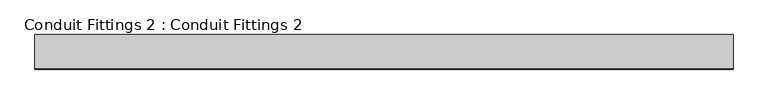
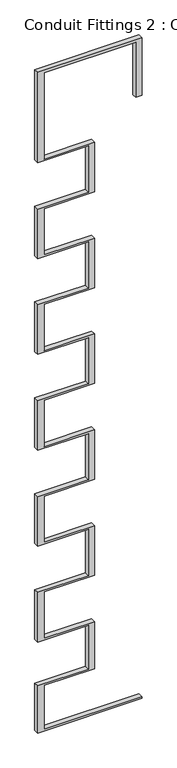
"""IFC4 building model written with IfcOpenShell, lengths in millimetres: cable carrier fitting geometry, Conduit Fittings 2 : Conduit Fittings 2."""

from ifc_helpers import new_model, si_unit, frame, origin, place, context, project, spatial, polyline, outline, extrude, source, transform, mapped, element, save


def conduit_fittings_2_conduit_fittings_2_af195c82(model_context):
    return source(origin(), model_context, "Body", "SweptSolid", [
        extrude(outline(polyline([(2946.4, -3622.597125), (3048.0, -3622.597125), (3048.0, -9528.097125), (5842.0, -9528.097125), (5842.0, -6480.097125), (8839.2, -6480.097125), (8839.2, -9528.097125), (11785.6, -9528.097125), (11785.6, -6480.097125), (14935.2, -6480.097125), (14935.2, -9534.447125), (17881.6, -9534.447125), (17881.6, -6480.097125), (21031.2, -6480.097125), (21031.2, -9528.097125), (23977.6, -9528.097125), (23977.6, -6480.097125), (27127.2, -6480.097125), (27127.2, -9534.447125), (30073.6, -9534.447125), (30073.6, -6480.097125), (33223.2, -6480.097125), (33223.2, -9534.447125), (36169.6, -9534.447125), (36169.6, -6480.097125), (39319.2, -6480.097125), (39319.2, -9528.097125), (44805.6, -9528.097125), (44805.6, -4003.597125), (41300.4, -4003.597125), (41300.4, -3622.597125), (44958.0, -3622.597125), (44958.0, -9909.097125), (39217.6, -9909.097125), (39217.6, -6854.747125), (36271.2, -6854.747125), (36271.2, -9909.097125), (33121.6, -9909.097125), (33121.6, -6861.097125), (30175.2, -6861.097125), (30175.2, -9909.097125), (27025.6, -9909.097125), (27025.6, -6861.097125), (24079.2, -6861.097125), (24079.2, -9909.097125), (20929.6, -9909.097125), (20929.6, -6861.097125), (17983.2, -6861.097125), (17983.2, -9909.097125), (14833.6, -9909.097125), (14833.6, -6861.097125), (11887.2, -6861.097125), (11887.2, -9909.097125), (8737.6, -9909.097125), (8737.6, -6861.097125), (5943.6, -6861.097125), (5943.6, -9909.097125), (2946.4, -9909.097125), (2946.4, -3622.597125)])), frame((0.0, -676.0934478, 0.0), z_axis=(0.0, 1.0, 0.0), x_axis=(0.0, 0.0, 1.0)), (0.0, 0.0, 1.0), 304.8),
    ])


if __name__ == "__main__":
    model = new_model("IFC4")
    model_context = context("Model", 3, world=origin())
    ifc_project = project(units=[si_unit("LENGTHUNIT", "METRE", prefix="MILLI")], contexts=[model_context])
    site = spatial("IfcSite", under=ifc_project)
    building = spatial("IfcBuilding", under=site)
    placement = place(None, origin())
    conduit_fittings_2_conduit_fittings_2_shape = conduit_fittings_2_conduit_fittings_2_af195c82(model_context)
    element("IfcCableCarrierFitting", 1, ObjectType="Conduit Fittings 2 : Conduit Fittings 2", at=placement, inside=building, context=model_context, shape_type="MappedRepresentation", body=[
        mapped(conduit_fittings_2_conduit_fittings_2_shape, transform((0.0, 0.0, 0.0), x_axis=(1.0, 0.0, 0.0), y_axis=(0.0, 1.0, 0.0), z_axis=(0.0, 0.0, 1.0))),
    ])
    save(model, "model.ifc")
